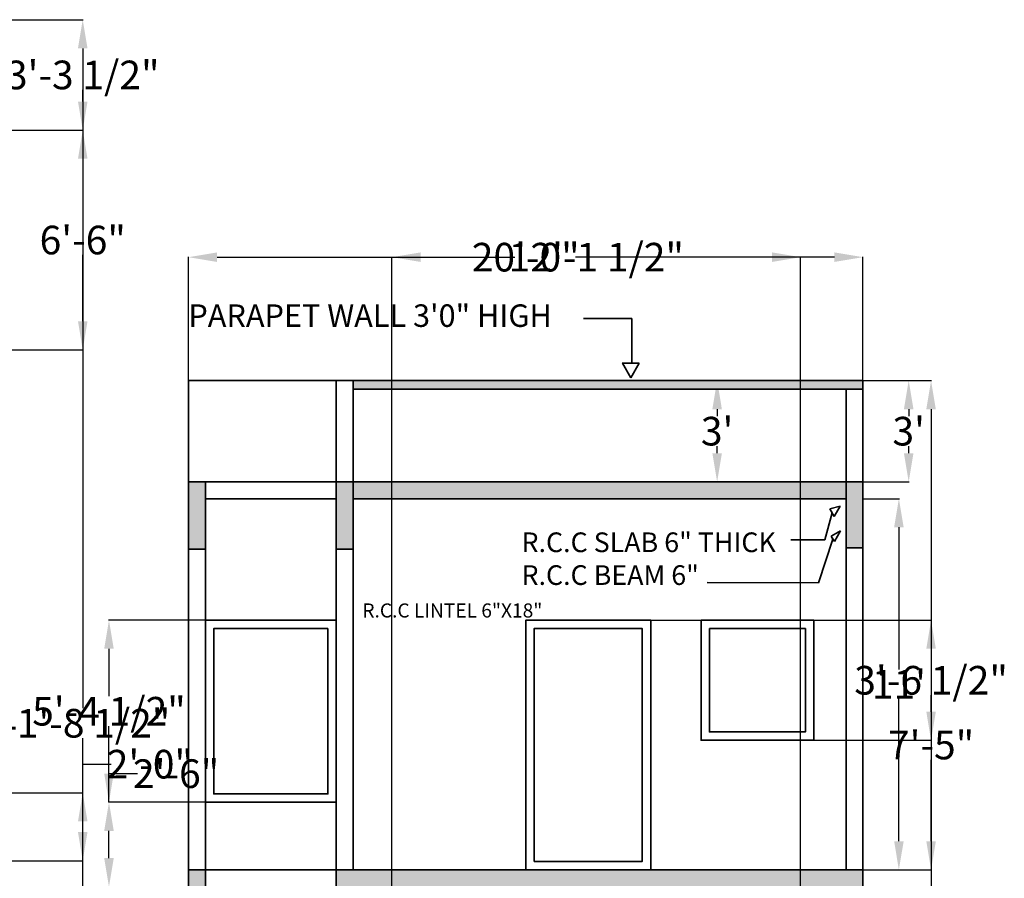
# Model space of a CAD drawing. Units: inches. Extents: x 21 to 3450, y 4 to 2137.
# Tile 8 of 14: x 2431 to 2781, y 1790 to 2095. Entities that reach past the tile are written whole.
import ezdxf

# ---------------------------------------------------------------- set-up
doc = ezdxf.new("R2010")
doc.units = ezdxf.units.IN
doc.header["$MEASUREMENT"] = 0
for name, color, linetype, lineweight in [('A-ANNO-DIMS', 2, 'Continuous', 18), ('A-ANNO-TEXT', 7, 'Continuous', 18), ('A-SECT', 7, 'Continuous', 35), ('A-SECT-PATT', 8, 'Continuous', 13)]:
    doc.layers.add(name, color=color, linetype=linetype, lineweight=lineweight)
doc.styles.get("Standard").update_dxf_attribs({"font": 'arial.ttf'})
doc.dimstyles.get("Standard").update_dxf_attribs({"dimtxt": 10.18, "dimasz": 10.18, "dimexe": 0.18, "dimexo": 0.0625, "dimgap": 0.09, "dimtad": 0, "dimtih": 1, "dimtoh": 1, "dimdec": 0, "dimzin": 0, "dimdsep": 46, "dimlunit": 3, "dimtxsty": 'Standard', "dimcen": 0.09, "dimadec": 0, "dimazin": 0, "dimtfac": 1, "dimtdec": 0, "dimtofl": 0, "dimtmove": 0, "dimatfit": 3, "dimfxl": 1, "dimtolj": 1, "dimtzin": 0, "dimarcsym": 0})

# ---------------------------------------------------------------- blocks, each defined once
blk = doc.blocks.new('*D11')
at = {"layer": 'A-ANNO-DIMS', "color": 0, "lineweight": -2, "transparency": 16777216}
for p, q in [((2685.18, 1966.57), (2679, 1966.57)), ((2679.18, 1956.39), (2679.18, 1953.86)), ((2679.18, 1940.75), (2679.18, 1943.27)), ((2685.18, 1930.57), (2679, 1930.57))]:
    blk.add_line(p, q, dxfattribs=at)
at = {"layer": 'A-ANNO-DIMS', "color": 0, "transparency": 16777216}
for points in [[(2677.48, 1956.39), (2680.87, 1956.39), (2679.18, 1966.57)], [(2677.48, 1940.75), (2680.87, 1940.75), (2679.18, 1930.57)]]:
    blk.add_solid(points, dxfattribs=at)
at = {"layer": 'Defpoints', "color": 0, "transparency": 16777216}
for p in [(2679.18, 1966.57), (2685.24, 1966.57), (2685.24, 1930.57)]:
    blk.add_point(p, dxfattribs=at)
at = {"layer": 'A-ANNO-DIMS', "color": 0, "transparency": 16777216, "insert": (2679.18, 1948.57), "char_height": 10.18, "attachment_point": 5}
blk.add_mtext("\\A1;3'", dxfattribs=at)
blk = doc.blocks.new('*D14')
at = {"layer": 'A-ANNO-DIMS', "color": 0, "lineweight": -2, "transparency": 16777216}
for p, q in [((2731.13, 1924.57), (2744.03, 1924.57)), ((2743.85, 1914.39), (2743.85, 1863.77)), ((2743.85, 1802.75), (2743.85, 1853.37)), ((2731.13, 1792.57), (2744.03, 1792.57))]:
    blk.add_line(p, q, dxfattribs=at)
at = {"layer": 'A-ANNO-DIMS', "color": 0, "transparency": 16777216}
for points in [[(2742.16, 1914.39), (2745.55, 1914.39), (2743.85, 1924.57)], [(2742.16, 1802.75), (2745.55, 1802.75), (2743.85, 1792.57)]]:
    blk.add_solid(points, dxfattribs=at)
at = {"layer": 'Defpoints', "color": 0, "transparency": 16777216}
for p in [(2731.07, 1924.57), (2743.85, 1924.57), (2731.07, 1792.57)]:
    blk.add_point(p, dxfattribs=at)
at = {"layer": 'A-ANNO-DIMS', "color": 0, "transparency": 16777216, "insert": (2743.85, 1858.57), "char_height": 10.18, "attachment_point": 5}
blk.add_mtext("\\A1;11'", dxfattribs=at)
blk = doc.blocks.new('*D15')
at = {"layer": 'A-ANNO-DIMS', "color": 0, "lineweight": -2, "transparency": 16777216}
for p, q in [((2731.13, 1966.57), (2747.52, 1966.57)), ((2747.34, 1956.39), (2747.34, 1953.86)), ((2747.34, 1940.75), (2747.34, 1943.27)), ((2731.13, 1930.57), (2747.52, 1930.57))]:
    blk.add_line(p, q, dxfattribs=at)
at = {"layer": 'A-ANNO-DIMS', "color": 0, "transparency": 16777216}
for points in [[(2745.65, 1956.39), (2749.04, 1956.39), (2747.34, 1966.57)], [(2745.65, 1940.75), (2749.04, 1940.75), (2747.34, 1930.57)]]:
    blk.add_solid(points, dxfattribs=at)
at = {"layer": 'Defpoints', "color": 0, "transparency": 16777216}
for p in [(2731.07, 1966.57), (2747.34, 1966.57), (2731.07, 1930.57)]:
    blk.add_point(p, dxfattribs=at)
at = {"layer": 'A-ANNO-DIMS', "color": 0, "transparency": 16777216, "insert": (2747.34, 1948.57), "char_height": 10.18, "attachment_point": 5}
blk.add_mtext("\\A1;3'", dxfattribs=at)
blk = doc.blocks.new('*D152')
at = {"layer": 'A-ANNO-DIMS', "color": 0, "lineweight": -2, "transparency": 16777216}
for p, q in [((2426.25, 2094.9), (2453.61, 2094.9)), ((2453.43, 2084.72), (2453.43, 1850.06)), ((2453.43, 1604.7), (2453.43, 1839.36)), ((2426.25, 1594.52), (2453.61, 1594.52))]:
    blk.add_line(p, q, dxfattribs=at)
at = {"layer": 'A-ANNO-DIMS', "color": 0, "transparency": 16777216}
for points in [[(2451.74, 2084.72), (2455.13, 2084.72), (2453.43, 2094.9)], [(2451.74, 1604.7), (2455.13, 1604.7), (2453.43, 1594.52)]]:
    blk.add_solid(points, dxfattribs=at)
at = {"layer": 'Defpoints', "color": 0, "transparency": 16777216}
for p in [(2426.18, 2094.9), (2453.43, 2094.9), (2426.18, 1594.52)]:
    blk.add_point(p, dxfattribs=at)
at = {"layer": 'A-ANNO-DIMS', "color": 0, "transparency": 16777216, "insert": (2453.43, 1844.71), "char_height": 10.18, "attachment_point": 5}
blk.add_mtext('\\A1;41\'-8 1/2"', dxfattribs=at)
blk = doc.blocks.new('*D159')
at = {"layer": 'A-ANNO-DIMS', "color": 0, "lineweight": -2, "transparency": 16777216}
for p, q in [((2426.25, 2055.62), (2453.61, 2055.62)), ((2453.43, 2045.44), (2453.43, 2021.84)), ((2453.43, 1987.67), (2453.43, 2011.27)), ((2426.25, 1977.49), (2453.61, 1977.49))]:
    blk.add_line(p, q, dxfattribs=at)
at = {"layer": 'A-ANNO-DIMS', "color": 0, "transparency": 16777216}
for points in [[(2451.74, 2045.44), (2455.13, 2045.44), (2453.43, 2055.62)], [(2451.74, 1987.67), (2455.13, 1987.67), (2453.43, 1977.49)]]:
    blk.add_solid(points, dxfattribs=at)
at = {"layer": 'Defpoints', "color": 0, "transparency": 16777216}
for p in [(2426.18, 2055.62), (2453.43, 2055.62), (2426.18, 1977.49)]:
    blk.add_point(p, dxfattribs=at)
at = {"layer": 'A-ANNO-DIMS', "color": 0, "transparency": 16777216, "insert": (2453.43, 2016.55), "char_height": 10.18, "attachment_point": 5}
blk.add_mtext('\\A1;6\'-6"', dxfattribs=at)
blk = doc.blocks.new('*D160')
at = {"layer": 'A-ANNO-DIMS', "color": 0, "lineweight": -2, "transparency": 16777216}
for p, q in [((2426.25, 2094.9), (2453.61, 2094.9)), ((2453.43, 2084.72), (2453.43, 2080.62)), ((2453.43, 2065.8), (2453.43, 2069.91)), ((2426.25, 2055.62), (2453.61, 2055.62))]:
    blk.add_line(p, q, dxfattribs=at)
at = {"layer": 'A-ANNO-DIMS', "color": 0, "transparency": 16777216}
for points in [[(2451.74, 2084.72), (2455.13, 2084.72), (2453.43, 2094.9)], [(2451.74, 2065.8), (2455.13, 2065.8), (2453.43, 2055.62)]]:
    blk.add_solid(points, dxfattribs=at)
at = {"layer": 'Defpoints', "color": 0, "transparency": 16777216}
for p in [(2426.18, 2094.9), (2453.43, 2094.9), (2426.18, 2055.62)]:
    blk.add_point(p, dxfattribs=at)
at = {"layer": 'A-ANNO-DIMS', "color": 0, "transparency": 16777216, "insert": (2453.43, 2075.26), "char_height": 10.18, "attachment_point": 5}
blk.add_mtext('\\A1;3\'-3 1/2"', dxfattribs=at)
blk = doc.blocks.new('*D176')
at = {"layer": 'A-ANNO-DIMS', "color": 0, "lineweight": -2, "transparency": 16777216}
for p, q in [((2453.43, 1819.97), (2453.43, 1830.15)), ((2453.43, 1830.15), (2463.61, 1830.15)), ((2306.25, 1819.97), (2453.61, 1819.97)), ((2453.43, 1805.98), (2453.43, 1809.79)), ((2306.25, 1795.8), (2453.61, 1795.8))]:
    blk.add_line(p, q, dxfattribs=at)
at = {"layer": 'A-ANNO-DIMS', "color": 0, "transparency": 16777216}
for points in [[(2451.74, 1809.79), (2455.13, 1809.79), (2453.43, 1819.97)], [(2451.74, 1805.98), (2455.13, 1805.98), (2453.43, 1795.8)]]:
    blk.add_solid(points, dxfattribs=at)
at = {"layer": 'Defpoints', "color": 0, "transparency": 16777216}
for p in [(2306.18, 1819.97), (2453.43, 1819.97), (2306.18, 1795.8)]:
    blk.add_point(p, dxfattribs=at)
at = {"layer": 'A-ANNO-DIMS', "color": 0, "transparency": 16777216, "insert": (2477.32, 1830.15), "char_height": 10.18, "attachment_point": 5}
blk.add_mtext('\\A1;2\'-0"', dxfattribs=at)
blk = doc.blocks.new('*D177')
at = {"layer": 'A-ANNO-DIMS', "color": 0, "lineweight": -2, "transparency": 16777216}
for p, q in [((2491.07, 1966.63), (2491.07, 2010.63)), ((2501.25, 2010.45), (2593.41, 2010.45)), ((2720.89, 2010.45), (2628.73, 2010.45)), ((2731.07, 1966.63), (2731.07, 2010.63))]:
    blk.add_line(p, q, dxfattribs=at)
at = {"layer": 'A-ANNO-DIMS', "color": 0, "transparency": 16777216}
for points in [[(2501.25, 2012.15), (2501.25, 2008.75), (2491.07, 2010.45)], [(2720.89, 2012.15), (2720.89, 2008.75), (2731.07, 2010.45)]]:
    blk.add_solid(points, dxfattribs=at)
at = {"layer": 'Defpoints', "color": 0, "transparency": 16777216}
for p in [(2731.07, 2010.45), (2491.07, 1966.57), (2731.07, 1966.57)]:
    blk.add_point(p, dxfattribs=at)
at = {"layer": 'A-ANNO-DIMS', "color": 0, "transparency": 16777216, "insert": (2611.07, 2010.45), "char_height": 10.18, "attachment_point": 5}
blk.add_mtext('\\A1;20\'-0"', dxfattribs=at)
blk = doc.blocks.new('*D178')
at = {"layer": 'A-ANNO-DIMS', "color": 0, "lineweight": -2, "transparency": 16777216}
for p, q in [((2731.13, 1966.57), (2755.48, 1966.57)), ((2755.3, 1956.39), (2755.3, 1785.86)), ((2755.3, 1604.75), (2755.3, 1775.27)), ((2731.13, 1594.57), (2755.48, 1594.57))]:
    blk.add_line(p, q, dxfattribs=at)
at = {"layer": 'A-ANNO-DIMS', "color": 0, "transparency": 16777216}
for points in [[(2753.61, 1956.39), (2757, 1956.39), (2755.3, 1966.57)], [(2753.61, 1604.75), (2757, 1604.75), (2755.3, 1594.57)]]:
    blk.add_solid(points, dxfattribs=at)
at = {"layer": 'Defpoints', "color": 0, "transparency": 16777216}
for p in [(2731.07, 1966.57), (2755.3, 1966.57), (2731.07, 1594.57)]:
    blk.add_point(p, dxfattribs=at)
at = {"layer": 'A-ANNO-DIMS', "color": 0, "transparency": 16777216, "insert": (2755.3, 1780.57), "char_height": 10.18, "attachment_point": 5}
blk.add_mtext('\\A1;31\'-0"', dxfattribs=at)
blk = doc.blocks.new('*D189')
at = {"layer": 'A-ANNO-DIMS', "color": 0, "lineweight": -2, "transparency": 16777216}
for p, q in [((2462.77, 1816.6), (2462.77, 1826.78)), ((2462.77, 1826.78), (2472.95, 1826.78)), ((2543.58, 1816.6), (2462.59, 1816.6)), ((2462.77, 1796.75), (2462.77, 1806.42)), ((2543.58, 1786.57), (2462.59, 1786.57))]:
    blk.add_line(p, q, dxfattribs=at)
at = {"layer": 'A-ANNO-DIMS', "color": 0, "transparency": 16777216}
for points in [[(2461.07, 1806.42), (2464.47, 1806.42), (2462.77, 1816.6)], [(2461.07, 1796.75), (2464.47, 1796.75), (2462.77, 1786.57)]]:
    blk.add_solid(points, dxfattribs=at)
at = {"layer": 'Defpoints', "color": 0, "transparency": 16777216}
for p in [(2462.77, 1816.6), (2543.65, 1816.6), (2543.65, 1786.57)]:
    blk.add_point(p, dxfattribs=at)
at = {"layer": 'A-ANNO-DIMS', "color": 0, "transparency": 16777216, "insert": (2486.66, 1826.78), "char_height": 10.18, "attachment_point": 5}
blk.add_mtext('\\A1;2\'-6"', dxfattribs=at)
blk = doc.blocks.new('*D190')
at = {"layer": 'A-ANNO-DIMS', "color": 0, "lineweight": -2, "transparency": 16777216}
for p, q in [((2543.58, 1881.35), (2462.59, 1881.35)), ((2462.77, 1871.17), (2462.77, 1854.33)), ((2462.77, 1826.78), (2462.77, 1843.62)), ((2543.58, 1816.6), (2462.59, 1816.6))]:
    blk.add_line(p, q, dxfattribs=at)
at = {"layer": 'A-ANNO-DIMS', "color": 0, "transparency": 16777216}
for points in [[(2461.07, 1871.17), (2464.47, 1871.17), (2462.77, 1881.35)], [(2461.07, 1826.78), (2464.47, 1826.78), (2462.77, 1816.6)]]:
    blk.add_solid(points, dxfattribs=at)
at = {"layer": 'Defpoints', "color": 0, "transparency": 16777216}
for p in [(2462.77, 1881.35), (2543.65, 1881.35), (2543.65, 1816.6)]:
    blk.add_point(p, dxfattribs=at)
at = {"layer": 'A-ANNO-DIMS', "color": 0, "transparency": 16777216, "insert": (2462.77, 1848.97), "char_height": 10.18, "attachment_point": 5}
blk.add_mtext('\\A1;5\'-4 1/2"', dxfattribs=at)
blk = doc.blocks.new('*D191')
at = {"layer": 'A-ANNO-DIMS', "color": 0, "lineweight": -2, "transparency": 16777216}
for p, q in [((2655.62, 1881.35), (2755.48, 1881.35)), ((2755.3, 1871.17), (2755.3, 1842.22)), ((2755.3, 1802.75), (2755.3, 1831.69)), ((2655.62, 1792.57), (2755.48, 1792.57))]:
    blk.add_line(p, q, dxfattribs=at)
at = {"layer": 'A-ANNO-DIMS', "color": 0, "transparency": 16777216}
for points in [[(2753.61, 1871.17), (2757, 1871.17), (2755.3, 1881.35)], [(2753.61, 1802.75), (2757, 1802.75), (2755.3, 1792.57)]]:
    blk.add_solid(points, dxfattribs=at)
at = {"layer": 'Defpoints', "color": 0, "transparency": 16777216}
for p in [(2655.56, 1881.35), (2755.3, 1881.35), (2655.56, 1792.57)]:
    blk.add_point(p, dxfattribs=at)
at = {"layer": 'A-ANNO-DIMS', "color": 0, "transparency": 16777216, "insert": (2755.3, 1836.96), "char_height": 10.18, "attachment_point": 5}
blk.add_mtext('\\A1;7\'-5"', dxfattribs=at)
blk = doc.blocks.new('*D192')
at = {"layer": 'A-ANNO-DIMS', "color": 0, "lineweight": -2, "transparency": 16777216}
for p, q in [((2713.65, 1881.35), (2755.48, 1881.35)), ((2755.3, 1871.17), (2755.3, 1865.35)), ((2755.3, 1848.82), (2755.3, 1854.64)), ((2713.65, 1838.64), (2755.48, 1838.64))]:
    blk.add_line(p, q, dxfattribs=at)
at = {"layer": 'A-ANNO-DIMS', "color": 0, "transparency": 16777216}
for points in [[(2753.61, 1871.17), (2757, 1871.17), (2755.3, 1881.35)], [(2753.61, 1848.82), (2757, 1848.82), (2755.3, 1838.64)]]:
    blk.add_solid(points, dxfattribs=at)
at = {"layer": 'Defpoints', "color": 0, "transparency": 16777216}
for p in [(2713.58, 1881.35), (2755.3, 1881.35), (2713.58, 1838.64)]:
    blk.add_point(p, dxfattribs=at)
at = {"layer": 'A-ANNO-DIMS', "color": 0, "transparency": 16777216, "insert": (2755.3, 1859.99), "char_height": 10.18, "attachment_point": 5}
blk.add_mtext('\\A1;3\'-6 1/2"', dxfattribs=at)
blk = doc.blocks.new('*D194')
at = {"layer": 'A-ANNO-DIMS', "color": 0, "lineweight": -2, "transparency": 16777216}
for p, q in [((2563.48, 1599.19), (2563.48, 2010.63)), ((2573.66, 2010.45), (2607.24, 2010.45)), ((2698.72, 2010.45), (2665.15, 2010.45)), ((2708.9, 1599.19), (2708.9, 2010.63))]:
    blk.add_line(p, q, dxfattribs=at)
at = {"layer": 'A-ANNO-DIMS', "color": 0, "transparency": 16777216}
for points in [[(2573.66, 2012.15), (2573.66, 2008.75), (2563.48, 2010.45)], [(2698.72, 2012.15), (2698.72, 2008.75), (2708.9, 2010.45)]]:
    blk.add_solid(points, dxfattribs=at)
at = {"layer": 'Defpoints', "color": 0, "transparency": 16777216}
for p in [(2708.9, 2010.45), (2563.48, 1599.13), (2708.9, 1599.13)]:
    blk.add_point(p, dxfattribs=at)
at = {"layer": 'A-ANNO-DIMS', "color": 0, "transparency": 16777216, "insert": (2636.19, 2010.45), "char_height": 10.18, "attachment_point": 5}
blk.add_mtext('\\A1;12\'-1 1/2"', dxfattribs=at)

msp = doc.modelspace()

# ---------------------------------------------------------------- hatches: boundary and pattern name
at = {"layer": 'A-SECT-PATT'}
h = msp.add_hatch(color=256, dxfattribs=at)
h.dxf.hatch_style = 1
h.paths.add_polyline_path([(2725.07, 1966.57), (2549.65, 1966.57), (2549.65, 1963.57), (2725.07, 1963.57)])
h.paths.add_polyline_path([(2731.07, 1966.57), (2725.07, 1966.57), (2725.07, 1963.57), (2731.07, 1963.57)])
h = msp.add_hatch(color=256, dxfattribs=at)
h.dxf.hatch_style = 1
h.paths.add_polyline_path([(2731.07, 1930.57), (2543.65, 1930.57), (2543.65, 1924.57), (2543.65, 1906.57), (2549.65, 1906.57), (2549.65, 1924.57), (2725.07, 1924.57), (2725.07, 1907.07), (2731.07, 1907.07)])
h.paths.add_polyline_path([(2497.07, 1930.57), (2491.07, 1930.57), (2491.07, 1906.57), (2497.07, 1906.57)])
h = msp.add_hatch(color=256, dxfattribs=at)
h.dxf.hatch_style = 1
h.paths.add_polyline_path([(2731.07, 1792.57), (2725.07, 1792.57), (2543.65, 1792.57), (2543.65, 1770.05), (2549.65, 1770.05), (2549.65, 1786.57), (2725.07, 1786.57), (2725.07, 1770.05), (2731.07, 1770.05)])
h.paths.add_polyline_path([(2497.07, 1792.57), (2491.07, 1792.57), (2491.07, 1769.13), (2497.07, 1769.13)])

# ---------------------------------------------------------------- linework, layer by layer
at = {"layer": 'A-SECT'}
for p, q in [((2631.57, 1988.6), (2648.85, 1988.6)), ((2648.85, 1988.6), (2648.85, 1972.77)), ((2648.85, 1972.77), (2645.4, 1972.77)), ((2645.4, 1972.77), (2651.45, 1972.77)), ((2648.45, 1967.58), (2645.46, 1972.77)), ((2651.45, 1972.77), (2648.45, 1967.58)), ((2491.07, 1594.57), (2491.07, 1966.57)), ((2491.07, 1966.57), (2731.07, 1966.57)), ((2543.65, 1924.57), (2543.65, 1966.57)), ((2549.65, 1966.57), (2549.65, 1792.57)), ((2731.07, 1594.57), (2731.07, 1966.57)), ((2549.65, 1963.57), (2731.07, 1963.57)), ((2725.07, 1792.57), (2725.07, 1963.57)), ((2491.07, 1930.57), (2731.07, 1930.57)), ((2497.07, 1642.57), (2497.07, 1930.57)), ((2491.07, 1792.57), (2491.07, 1924.57)), ((2497.07, 1924.57), (2543.65, 1924.57)), ((2543.65, 1924.57), (2543.65, 1642.57)), ((2549.65, 1924.57), (2725.07, 1924.57)), ((2722.92, 1921.86), (2719.26, 1920.98)), ((2720.07, 1919.57), (2719.26, 1920.98)), ((2719.26, 1920.98), (2720.83, 1918.25)), ((2720.83, 1918.25), (2722.92, 1921.86)), ((2717.46, 1909.95), (2720.07, 1919.57)), ((2723.09, 1913.16), (2719.75, 1911.29)), ((2720.89, 1909.33), (2723.09, 1913.16)), ((2705.42, 1909.92), (2717.46, 1909.95)), ((2715.23, 1894.59), (2720.38, 1910.2)), ((2720.38, 1910.2), (2719.75, 1911.29)), ((2719.75, 1911.29), (2720.89, 1909.33)), ((2491.07, 1906.57), (2497.07, 1906.57)), ((2543.65, 1906.57), (2549.65, 1906.57)), ((2725.07, 1907.07), (2731.07, 1907.07)), ((2675.63, 1894.77), (2715.23, 1894.59)), ((2725.07, 1802.29), (2725.07, 1831.58)), ((2731.07, 1802.29), (2731.07, 1831.58)), ((2497.07, 1792.57), (2491.07, 1792.57)), ((2497.07, 1792.57), (2725.07, 1792.57)), ((2725.07, 1792.57), (2731.07, 1792.57))]:
    msp.add_line(p, q, dxfattribs=at)
for points in [[(2731.07, 1983.97), (2731.07, 1983.97)], [(2731.07, 1972.57), (2731.07, 1972.57)], [(2543.65, 1881.35), (2543.65, 1881.35), (2497.07, 1881.35), (2497.07, 1881.35), (2497.07, 1816.6), (2497.07, 1816.6), (2543.65, 1816.6), (2543.65, 1816.6)], [(2540.65, 1878.35), (2500.07, 1878.35), (2500.07, 1819.6), (2540.65, 1819.6)], [(2611.07, 1792.57), (2611.07, 1792.57), (2655.56, 1792.57), (2655.56, 1792.57), (2655.56, 1881.35), (2655.56, 1881.35), (2611.07, 1881.35), (2611.07, 1881.35)], [(2614.07, 1795.57), (2652.56, 1795.57), (2652.56, 1878.35), (2614.07, 1878.35)], [(2673.46, 1881.35), (2673.46, 1881.35), (2713.58, 1881.35), (2713.58, 1881.35), (2713.58, 1838.64), (2713.58, 1838.64), (2673.46, 1838.64), (2673.46, 1838.64)], [(2676.46, 1878.35), (2710.58, 1878.35), (2710.58, 1841.64), (2676.46, 1841.64)]]:
    msp.add_lwpolyline(points, close=True, dxfattribs=at)

# ---------------------------------------------------------------- texts
at = {"layer": 'A-ANNO-TEXT', "attachment_point": 1}
for s, width, insert, char_height in [('PARAPET WALL 3\'0" HIGH', 267.3822, (2491.02, 1993.66), 8), ('R.C.C SLAB 6" THICK \\PR.C.C BEAM 6"', 108.6091, (2609.56, 1912.56), 7), ('R.C.C LINTEL 6"X18"', 267.3822, (2552.93, 1887.31), 5)]:
    msp.add_mtext_dynamic_manual_height_columns(s, width=width, gutter_width=1, heights=[0], dxfattribs=dict(at, insert=insert, char_height=char_height))

# ---------------------------------------------------------------- dimensions: what is measured, and where the dimension line sits
at = {"layer": 'A-ANNO-DIMS'}
for base, p1, p2, override, picture, middle in [((2453.43, 2094.9), (2426.18, 1594.52), (2426.18, 2094.9), {"dimdec": 1, "dimlfac": 1, "dimrnd": 0, "dimzin": 1, "dimdsep": 46, "dimlunit": 4, "dimfrac": 2}, '*D152', (2453.43, 1844.71)), ((2453.43, 2094.9), (2426.18, 2055.62), (2426.18, 2094.9), {"dimdec": 1, "dimlfac": 1, "dimrnd": 0, "dimzin": 1, "dimdsep": 46, "dimlunit": 4, "dimfrac": 2}, '*D160', (2453.43, 2075.26)), ((2453.43, 2055.62), (2426.18, 1977.49), (2426.18, 2055.62), {"dimdec": 1, "dimlfac": 1, "dimrnd": 0, "dimzin": 1, "dimdsep": 46, "dimlunit": 4, "dimfrac": 2}, '*D159', (2453.43, 2016.55)), ((2679.18, 1966.57), (2685.24, 1930.57), (2685.24, 1966.57), {"dimclrd": 0, "dimclre": 0, "dimclrt": 0}, '*D11', (2679.18, 1948.57)), ((2747.34, 1966.57), (2731.07, 1930.57), (2731.07, 1966.57), {"dimclrd": 0, "dimclre": 0, "dimclrt": 0}, '*D15', (2747.34, 1948.57)), ((2755.3, 1966.57), (2731.07, 1594.57), (2731.07, 1966.57), {"dimdec": 1, "dimlfac": 1, "dimrnd": 0, "dimzin": 1, "dimdsep": 46, "dimlunit": 4, "dimfrac": 2}, '*D178', (2755.3, 1780.57)), ((2743.85, 1924.57), (2731.07, 1792.57), (2731.07, 1924.57), {"dimclrd": 0, "dimclre": 0, "dimclrt": 0}, '*D14', (2743.85, 1858.57)), ((2462.7694, 1881.3478), (2543.6453, 1816.6011), (2543.6453, 1881.3478), {"dimdec": 1, "dimlfac": 1, "dimrnd": 0, "dimzin": 1, "dimdsep": 46, "dimlunit": 4, "dimfrac": 2}, '*D190', (2462.7694, 1848.9744)), ((2755.3, 1881.35), (2655.56, 1792.57), (2655.56, 1881.35), {"dimdec": 1, "dimlfac": 1, "dimrnd": 0, "dimzin": 1, "dimdsep": 46, "dimlunit": 4, "dimfrac": 2}, '*D191', (2755.3, 1836.96)), ((2755.3, 1881.35), (2713.58, 1838.64), (2713.58, 1881.35), {"dimdec": 1, "dimlfac": 1, "dimrnd": 0, "dimzin": 1, "dimdsep": 46, "dimlunit": 4, "dimfrac": 2}, '*D192', (2755.3, 1859.99)), ((2453.43, 1819.97), (2306.18, 1795.8), (2306.18, 1819.97), {"dimdec": 1, "dimlfac": 1, "dimrnd": 0, "dimzin": 1, "dimdsep": 46, "dimlunit": 4, "dimfrac": 2}, '*D176', (2477.32, 1830.15)), ((2462.77, 1816.6), (2543.65, 1786.57), (2543.65, 1816.6), {"dimdec": 1, "dimlfac": 1, "dimrnd": 0, "dimzin": 1, "dimdsep": 46, "dimlunit": 4, "dimfrac": 2}, '*D189', (2486.66, 1826.78))]:
    dim = msp.add_linear_dim(base=base, p1=p1, p2=p2, angle=90, dimstyle='Standard', override=override, dxfattribs=at)
    dim.commit()
    dim.dimension.update_dxf_attribs({"geometry": picture, "text_midpoint": middle})
for base, p1, p2, picture, middle in [((2708.9, 2010.45), (2563.48, 1599.13), (2708.9, 1599.13), '*D194', (2636.19, 2010.45)), ((2731.07, 2010.45), (2491.07, 1966.57), (2731.07, 1966.57), '*D177', (2611.07, 2010.45))]:
    dim = msp.add_linear_dim(base=base, p1=p1, p2=p2, dimstyle='Standard', override={"dimdec": 1, "dimlfac": 1, "dimrnd": 0, "dimzin": 1, "dimdsep": 46, "dimlunit": 4, "dimfrac": 2}, dxfattribs=at)
    dim.commit()
    dim.dimension.update_dxf_attribs({"geometry": picture, "text_midpoint": middle})

doc.saveas('drawing.dxf')
